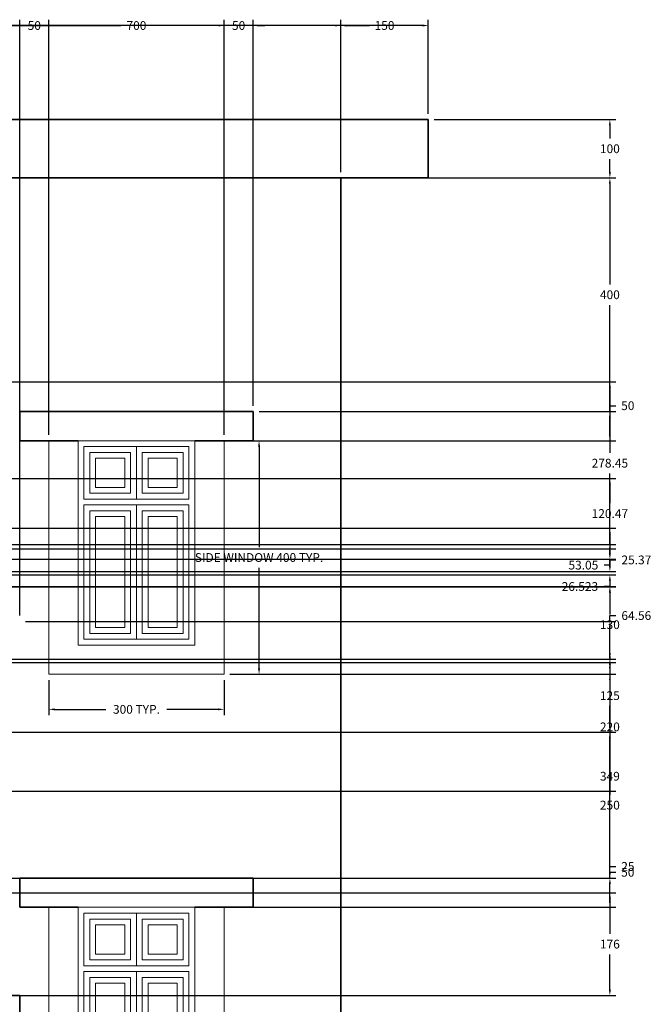
# Model space of a CAD drawing. Units: millimetres. Extents: x 937 to 4561, y 2711 to 5748.
# Tile 8 of 8: x 3479 to 4561, y 4062 to 5748. Entities that reach past the tile are written whole.
import ezdxf

# ---------------------------------------------------------------- set-up
doc = ezdxf.new("R2010")
doc.units = ezdxf.units.MM
doc.header["$MEASUREMENT"] = 0
for name, color, linetype, lineweight in [('A-ANNO-DIMS', 2, 'Continuous', 18), ('A-ELEV', 7, 'Continuous', 35), ('A-GLAZ', 4, 'Continuous', 18)]:
    doc.layers.add(name, color=color, linetype=linetype, lineweight=lineweight)
doc.styles.get("Standard").update_dxf_attribs({"font": 'arial.ttf'})
doc.dimstyles.get("Standard").update_dxf_attribs({"dimtxt": 15, "dimasz": 10, "dimexe": 10, "dimexo": 10, "dimgap": 10, "dimtad": 0, "dimtih": 1, "dimtoh": 1, "dimdec": 0, "dimzin": 0, "dimdsep": 46, "dimtxsty": 'Standard', "dimcen": 5, "dimadec": 0, "dimazin": 0, "dimtfac": 1, "dimtdec": 0, "dimtofl": 0, "dimtmove": 0, "dimatfit": 3, "dimfxl": 1, "dimtolj": 1, "dimtzin": 0, "dimarcsym": 0})

# ---------------------------------------------------------------- blocks, each defined once
blk = doc.blocks.new('WIN-SIDE')
for p, q in [((3529.5, 5026.9), (3529.5, 4626.9)), ((3579.5, 5026.9), (3779.5, 5026.9)), ((3579.5, 4676.9), (3579.5, 5026.9)), ((3779.5, 5026.9), (3779.5, 4676.9)), ((3829.5, 4626.9), (3829.5, 5026.9)), ((3779.5, 4676.9), (3579.5, 4676.9)), ((3529.5, 4626.9), (3829.5, 4626.9))]:
    blk.add_line(p, q)
for points in [[(3589.5, 5016.9), (3679.5, 5016.9), (3679.5, 4926.9), (3589.5, 4926.9)], [(3679.5, 5016.9), (3769.5, 5016.9), (3769.5, 4926.9), (3679.5, 4926.9)], [(3599.5, 5006.9), (3669.5, 5006.9), (3669.5, 4936.9), (3599.5, 4936.9)], [(3609.5, 4996.9), (3659.5, 4996.9), (3659.5, 4946.9), (3609.5, 4946.9)], [(3689.5, 5006.9), (3759.5, 5006.9), (3759.5, 4936.9), (3689.5, 4936.9)], [(3699.5, 4996.9), (3749.5, 4996.9), (3749.5, 4946.9), (3699.5, 4946.9)], [(3589.5, 4916.9), (3679.5, 4916.9), (3679.5, 4686.9), (3589.5, 4686.9)], [(3599.5, 4906.9), (3669.5, 4906.9), (3669.5, 4696.9), (3599.5, 4696.9)], [(3679.5, 4916.9), (3769.5, 4916.9), (3769.5, 4686.9), (3679.5, 4686.9)], [(3689.5, 4906.9), (3759.5, 4906.9), (3759.5, 4696.9), (3689.5, 4696.9)], [(3609.5, 4896.9), (3659.5, 4896.9), (3659.5, 4706.9), (3609.5, 4706.9)], [(3699.5, 4896.9), (3749.5, 4896.9), (3749.5, 4706.9), (3699.5, 4706.9)]]:
    blk.add_lwpolyline(points, close=True)
blk = doc.blocks.new('*D2')
at = {"layer": 'A-ANNO-DIMS', "color": 0, "lineweight": -2, "transparency": 16777216}
for p, q in [((3839.5, 5026.9), (3899.5, 5026.9)), ((3889.5, 5016.9), (3889.5, 4844.7)), ((3889.5, 4636.9), (3889.5, 4809.1)), ((3839.5, 4626.9), (3899.5, 4626.9))]:
    blk.add_line(p, q, dxfattribs=at)
at = {"layer": 'A-ANNO-DIMS', "color": 0, "transparency": 16777216}
for points in [[(3887.8, 5016.9), (3891.2, 5016.9), (3889.5, 5026.9)], [(3887.8, 4636.9), (3891.2, 4636.9), (3889.5, 4626.9)]]:
    blk.add_solid(points, dxfattribs=at)
at = {"layer": 'Defpoints', "color": 0, "transparency": 16777216}
for p in [(3829.5, 5026.9), (3889.5, 5026.9), (3829.5, 4626.9)]:
    blk.add_point(p, dxfattribs=at)
at = {"layer": 'A-ANNO-DIMS', "color": 0, "transparency": 16777216, "insert": (3889.5, 4826.9), "char_height": 15, "attachment_point": 5}
blk.add_mtext('\\A1;SIDE WINDOW 400 TYP.', dxfattribs=at)
blk = doc.blocks.new('*D3')
at = {"layer": 'A-ANNO-DIMS', "color": 0, "lineweight": -2, "transparency": 16777216}
for p, q in [((3529.5, 4616.9), (3529.5, 4556.9)), ((3829.5, 4616.9), (3829.5, 4556.9)), ((3539.5, 4566.9), (3627.2, 4566.9)), ((3819.5, 4566.9), (3731.8, 4566.9))]:
    blk.add_line(p, q, dxfattribs=at)
at = {"layer": 'A-ANNO-DIMS', "color": 0, "transparency": 16777216}
for points in [[(3539.5, 4568.6), (3539.5, 4565.2), (3529.5, 4566.9)], [(3819.5, 4568.6), (3819.5, 4565.2), (3829.5, 4566.9)]]:
    blk.add_solid(points, dxfattribs=at)
at = {"layer": 'Defpoints', "color": 0, "transparency": 16777216}
for p in [(3529.5, 4626.9), (3829.5, 4626.9), (3829.5, 4566.9)]:
    blk.add_point(p, dxfattribs=at)
at = {"layer": 'A-ANNO-DIMS', "color": 0, "transparency": 16777216, "insert": (3679.5, 4566.9), "char_height": 15, "attachment_point": 5}
blk.add_mtext('\\A1;300 TYP.', dxfattribs=at)
blk = doc.blocks.new('*D15')
at = {"layer": 'A-ANNO-DIMS', "color": 0, "lineweight": -2, "transparency": 16777216}
for p, q in [((1329.5, 4086.9), (1329.5, 5747.9)), ((1339.5, 5737.9), (2722, 5737.9)), ((4169.5, 5737.9), (2787, 5737.9)), ((4179.5, 5586.9), (4179.5, 5747.9))]:
    blk.add_line(p, q, dxfattribs=at)
at = {"layer": 'A-ANNO-DIMS', "color": 0, "transparency": 16777216}
for points in [[(1339.5, 5739.6), (1339.5, 5736.2), (1329.5, 5737.9)], [(4169.5, 5739.6), (4169.5, 5736.2), (4179.5, 5737.9)]]:
    blk.add_solid(points, dxfattribs=at)
at = {"layer": 'Defpoints', "color": 0, "transparency": 16777216}
for p in [(4179.5, 5737.9), (4179.5, 5576.9), (1329.5, 4076.9)]:
    blk.add_point(p, dxfattribs=at)
at = {"layer": 'A-ANNO-DIMS', "color": 0, "transparency": 16777216, "insert": (2754.5, 5737.9), "char_height": 15, "attachment_point": 5}
blk.add_mtext('\\A1;2850', dxfattribs=at)
blk = doc.blocks.new('*D18')
at = {"layer": 'A-ANNO-DIMS', "color": 0, "lineweight": -2, "transparency": 16777216}
for p, q in [((3329.5, 5486.9), (3329.5, 5747.9)), ((3339.5, 5737.9), (3653, 5737.9)), ((4019.5, 5737.9), (3706, 5737.9)), ((4029.5, 5486.9), (4029.5, 5747.9))]:
    blk.add_line(p, q, dxfattribs=at)
at = {"layer": 'A-ANNO-DIMS', "color": 0, "transparency": 16777216}
for points in [[(3339.5, 5739.6), (3339.5, 5736.2), (3329.5, 5737.9)], [(4019.5, 5739.6), (4019.5, 5736.2), (4029.5, 5737.9)]]:
    blk.add_solid(points, dxfattribs=at)
at = {"layer": 'Defpoints', "color": 0, "transparency": 16777216}
for p in [(4029.5, 5737.9), (3329.5, 5476.9), (4029.5, 5476.9)]:
    blk.add_point(p, dxfattribs=at)
at = {"layer": 'A-ANNO-DIMS', "color": 0, "transparency": 16777216, "insert": (3679.5, 5737.9), "char_height": 15, "attachment_point": 5}
blk.add_mtext('\\A1;700', dxfattribs=at)
blk = doc.blocks.new('*D19')
at = {"layer": 'A-ANNO-DIMS', "color": 0, "lineweight": -2, "transparency": 16777216}
for p, q in [((4029.5, 5486.9), (4029.5, 5747.9)), ((4039.5, 5737.9), (4078.6, 5737.9)), ((4169.5, 5737.9), (4130.3, 5737.9)), ((4179.5, 5586.9), (4179.5, 5747.9))]:
    blk.add_line(p, q, dxfattribs=at)
at = {"layer": 'A-ANNO-DIMS', "color": 0, "transparency": 16777216}
for points in [[(4039.5, 5739.6), (4039.5, 5736.2), (4029.5, 5737.9)], [(4169.5, 5739.6), (4169.5, 5736.2), (4179.5, 5737.9)]]:
    blk.add_solid(points, dxfattribs=at)
at = {"layer": 'Defpoints', "color": 0, "transparency": 16777216}
for p in [(4179.5, 5737.9), (4179.5, 5576.9), (4029.5, 5476.9)]:
    blk.add_point(p, dxfattribs=at)
at = {"layer": 'A-ANNO-DIMS', "color": 0, "transparency": 16777216, "insert": (4104.5, 5737.9), "char_height": 15, "attachment_point": 5}
blk.add_mtext('\\A1;150', dxfattribs=at)
blk = doc.blocks.new('*D23')
at = {"layer": 'A-ANNO-DIMS', "color": 0, "lineweight": -2, "transparency": 16777216}
for p, q in [((3029.5, 4886.9), (3029.5, 5747.9)), ((3039.5, 5737.9), (3227.6, 5737.9)), ((3469.5, 5737.9), (3281.3, 5737.9)), ((3479.5, 4727.5), (3479.5, 5747.9))]:
    blk.add_line(p, q, dxfattribs=at)
at = {"layer": 'A-ANNO-DIMS', "color": 0, "transparency": 16777216}
for points in [[(3039.5, 5739.6), (3039.5, 5736.2), (3029.5, 5737.9)], [(3469.5, 5739.6), (3469.5, 5736.2), (3479.5, 5737.9)]]:
    blk.add_solid(points, dxfattribs=at)
at = {"layer": 'Defpoints', "color": 0, "transparency": 16777216}
for p in [(3479.5, 5737.9), (3029.5, 4876.9), (3479.5, 4717.5)]:
    blk.add_point(p, dxfattribs=at)
at = {"layer": 'A-ANNO-DIMS', "color": 0, "transparency": 16777216, "insert": (3254.5, 5737.9), "char_height": 15, "attachment_point": 5}
blk.add_mtext('\\A1;450', dxfattribs=at)
blk = doc.blocks.new('*D25')
at = {"layer": 'A-ANNO-DIMS', "color": 0, "lineweight": -2, "transparency": 16777216}
for p, q in [((3469.5, 5737.9), (3459.5, 5737.9)), ((3479.5, 5086.9), (3479.5, 5747.9)), ((3529.5, 5036.9), (3529.5, 5747.9)), ((3539.5, 5737.9), (3549.5, 5737.9))]:
    blk.add_line(p, q, dxfattribs=at)
at = {"layer": 'A-ANNO-DIMS', "color": 0, "transparency": 16777216}
for points in [[(3469.5, 5739.6), (3469.5, 5736.2), (3479.5, 5737.9)], [(3539.5, 5739.6), (3539.5, 5736.2), (3529.5, 5737.9)]]:
    blk.add_solid(points, dxfattribs=at)
at = {"layer": 'Defpoints', "color": 0, "transparency": 16777216}
for p in [(3529.5, 5737.9), (3479.5, 5076.9), (3529.5, 5026.9)]:
    blk.add_point(p, dxfattribs=at)
at = {"layer": 'A-ANNO-DIMS', "color": 0, "transparency": 16777216, "insert": (3504.5, 5737.9), "char_height": 15, "attachment_point": 5}
blk.add_mtext('\\A1;50', dxfattribs=at)
blk = doc.blocks.new('*D26')
at = {"layer": 'A-ANNO-DIMS', "color": 0, "lineweight": -2, "transparency": 16777216}
for p, q in [((3819.5, 5737.9), (3809.5, 5737.9)), ((3829.5, 5036.9), (3829.5, 5747.9)), ((3879.5, 5086.9), (3879.5, 5747.9)), ((3889.5, 5737.9), (3899.5, 5737.9))]:
    blk.add_line(p, q, dxfattribs=at)
at = {"layer": 'A-ANNO-DIMS', "color": 0, "transparency": 16777216}
for points in [[(3819.5, 5739.6), (3819.5, 5736.2), (3829.5, 5737.9)], [(3889.5, 5739.6), (3889.5, 5736.2), (3879.5, 5737.9)]]:
    blk.add_solid(points, dxfattribs=at)
at = {"layer": 'Defpoints', "color": 0, "transparency": 16777216}
for p in [(3879.5, 5737.9), (3879.5, 5076.9), (3829.5, 5026.9)]:
    blk.add_point(p, dxfattribs=at)
at = {"layer": 'A-ANNO-DIMS', "color": 0, "transparency": 16777216, "insert": (3854.5, 5737.9), "char_height": 15, "attachment_point": 5}
blk.add_mtext('\\A1;50', dxfattribs=at)
blk = doc.blocks.new('*D68')
at = {"layer": 'A-ANNO-DIMS', "color": 0, "lineweight": -2, "transparency": 16777216}
for p, q in [((4490.5, 4812.8), (4490.5, 4822.8)), ((4490.5, 4822.8), (4500.5, 4822.8)), ((1364.5, 4802.8), (4500.5, 4802.8)), ((1364.5, 4777.4), (4500.5, 4777.4)), ((4490.5, 4767.4), (4490.5, 4757.4))]:
    blk.add_line(p, q, dxfattribs=at)
at = {"layer": 'A-ANNO-DIMS', "color": 0, "transparency": 16777216}
for points in [[(4488.8, 4812.8), (4492.2, 4812.8), (4490.5, 4802.8)], [(4488.8, 4767.4), (4492.2, 4767.4), (4490.5, 4777.4)]]:
    blk.add_solid(points, dxfattribs=at)
at = {"layer": 'Defpoints', "color": 0, "transparency": 16777216}
for p in [(1354.5, 4802.8), (4490.5, 4802.8), (1354.5, 4777.4)]:
    blk.add_point(p, dxfattribs=at)
at = {"layer": 'A-ANNO-DIMS', "color": 0, "transparency": 16777216, "insert": (4535.9, 4822.8), "char_height": 15, "attachment_point": 5}
blk.add_mtext('\\A1;25.37', dxfattribs=at)
blk = doc.blocks.new('*D69')
at = {"layer": 'A-ANNO-DIMS', "color": 0, "lineweight": -2, "transparency": 16777216}
for p, q in [((2957.4, 5127.7), (4500.5, 5127.7)), ((4490.5, 5117.7), (4490.5, 5006.1)), ((4490.5, 4859.2), (4490.5, 4970.8)), ((1339.5, 4849.2), (4500.5, 4849.2))]:
    blk.add_line(p, q, dxfattribs=at)
at = {"layer": 'A-ANNO-DIMS', "color": 0, "transparency": 16777216}
for points in [[(4488.8, 5117.7), (4492.2, 5117.7), (4490.5, 5127.7)], [(4488.8, 4859.2), (4492.2, 4859.2), (4490.5, 4849.2)]]:
    blk.add_solid(points, dxfattribs=at)
at = {"layer": 'Defpoints', "color": 0, "transparency": 16777216}
for p in [(2947.4, 5127.7), (4490.5, 5127.7), (1329.5, 4849.2)]:
    blk.add_point(p, dxfattribs=at)
at = {"layer": 'A-ANNO-DIMS', "color": 0, "transparency": 16777216, "insert": (4490.5, 4988.5), "char_height": 15, "attachment_point": 5}
blk.add_mtext('\\A1;278.45', dxfattribs=at)
blk = doc.blocks.new('*D75')
at = {"layer": 'A-ANNO-DIMS', "color": 0, "lineweight": -2, "transparency": 16777216}
for p, q in [((1829.5, 4646.9), (4500.5, 4646.9)), ((4490.5, 4636.9), (4490.5, 4554.6)), ((4490.5, 4436.9), (4490.5, 4519.2)), ((1829.5, 4426.9), (4500.5, 4426.9))]:
    blk.add_line(p, q, dxfattribs=at)
at = {"layer": 'A-ANNO-DIMS', "color": 0, "transparency": 16777216}
for points in [[(4488.8, 4636.9), (4492.2, 4636.9), (4490.5, 4646.9)], [(4488.8, 4436.9), (4492.2, 4436.9), (4490.5, 4426.9)]]:
    blk.add_solid(points, dxfattribs=at)
at = {"layer": 'Defpoints', "color": 0, "transparency": 16777216}
for p in [(1819.5, 4646.9), (4490.5, 4646.9), (1819.5, 4426.9)]:
    blk.add_point(p, dxfattribs=at)
at = {"layer": 'A-ANNO-DIMS', "color": 0, "transparency": 16777216, "insert": (4490.5, 4536.9), "char_height": 15, "attachment_point": 5}
blk.add_mtext('\\A1;220', dxfattribs=at)
blk = doc.blocks.new('*D76')
at = {"layer": 'A-ANNO-DIMS', "color": 0, "lineweight": -2, "transparency": 16777216}
for p, q in [((1829.5, 4776.9), (4500.5, 4776.9)), ((4490.5, 4766.9), (4490.5, 4729.6)), ((4490.5, 4656.9), (4490.5, 4694.2)), ((1829.5, 4646.9), (4500.5, 4646.9))]:
    blk.add_line(p, q, dxfattribs=at)
at = {"layer": 'A-ANNO-DIMS', "color": 0, "transparency": 16777216}
for points in [[(4488.8, 4766.9), (4492.2, 4766.9), (4490.5, 4776.9)], [(4488.8, 4656.9), (4492.2, 4656.9), (4490.5, 4646.9)]]:
    blk.add_solid(points, dxfattribs=at)
at = {"layer": 'Defpoints', "color": 0, "transparency": 16777216}
for p in [(1819.5, 4776.9), (4490.5, 4776.9), (1819.5, 4646.9)]:
    blk.add_point(p, dxfattribs=at)
at = {"layer": 'A-ANNO-DIMS', "color": 0, "transparency": 16777216, "insert": (4490.5, 4711.9), "char_height": 15, "attachment_point": 5}
blk.add_mtext('\\A1;130', dxfattribs=at)
blk = doc.blocks.new('*D78')
at = {"layer": 'A-ANNO-DIMS', "color": 0, "lineweight": -2, "transparency": 16777216}
for p, q in [((2439.5, 4962.4), (4500.5, 4962.4)), ((4490.5, 4952.4), (4490.5, 4919.9)), ((4490.5, 4852), (4490.5, 4884.5)), ((1739.5, 4842), (4500.5, 4842))]:
    blk.add_line(p, q, dxfattribs=at)
at = {"layer": 'A-ANNO-DIMS', "color": 0, "transparency": 16777216}
for points in [[(4488.8, 4952.4), (4492.2, 4952.4), (4490.5, 4962.4)], [(4488.8, 4852), (4492.2, 4852), (4490.5, 4842)]]:
    blk.add_solid(points, dxfattribs=at)
at = {"layer": 'Defpoints', "color": 0, "transparency": 16777216}
for p in [(2429.5, 4962.4), (4490.5, 4962.4), (1729.5, 4842)]:
    blk.add_point(p, dxfattribs=at)
at = {"layer": 'A-ANNO-DIMS', "color": 0, "transparency": 16777216, "insert": (4490.5, 4902.2), "char_height": 15, "attachment_point": 5}
blk.add_mtext('\\A1;120.47', dxfattribs=at)
blk = doc.blocks.new('*D80')
at = {"layer": 'A-ANNO-DIMS', "color": 0, "lineweight": -2, "transparency": 16777216}
for p, q in [((3039.5, 4876.9), (4500.5, 4876.9)), ((4490.5, 4866.9), (4490.5, 4833.9)), ((3039.5, 4823.9), (4500.5, 4823.9)), ((4490.5, 4823.9), (4490.5, 4813.9)), ((4490.5, 4813.9), (4480.5, 4813.9))]:
    blk.add_line(p, q, dxfattribs=at)
at = {"layer": 'A-ANNO-DIMS', "color": 0, "transparency": 16777216}
for points in [[(4488.8, 4866.9), (4492.2, 4866.9), (4490.5, 4876.9)], [(4488.8, 4833.9), (4492.2, 4833.9), (4490.5, 4823.9)]]:
    blk.add_solid(points, dxfattribs=at)
at = {"layer": 'Defpoints', "color": 0, "transparency": 16777216}
for p in [(3029.5, 4876.9), (3029.5, 4823.9), (4490.5, 4823.9)]:
    blk.add_point(p, dxfattribs=at)
at = {"layer": 'A-ANNO-DIMS', "color": 0, "transparency": 16777216, "insert": (4445.1, 4813.9), "char_height": 15, "attachment_point": 5}
blk.add_mtext('\\A1;53.05', dxfattribs=at)
blk = doc.blocks.new('*D81')
at = {"layer": 'A-ANNO-DIMS', "color": 0, "lineweight": -2, "transparency": 16777216}
for p, q in [((4490.5, 4833.9), (4490.5, 4843.9)), ((3039.5, 4823.9), (4500.5, 4823.9)), ((3039.5, 4797.3), (4500.5, 4797.3)), ((4490.5, 4777.3), (4480.5, 4777.3)), ((4490.5, 4787.3), (4490.5, 4777.3))]:
    blk.add_line(p, q, dxfattribs=at)
at = {"layer": 'A-ANNO-DIMS', "color": 0, "transparency": 16777216}
for points in [[(4488.8, 4833.9), (4492.2, 4833.9), (4490.5, 4823.9)], [(4488.8, 4787.3), (4492.2, 4787.3), (4490.5, 4797.3)]]:
    blk.add_solid(points, dxfattribs=at)
at = {"layer": 'Defpoints', "color": 0, "transparency": 16777216}
for p in [(3029.5, 4823.9), (3029.5, 4797.3), (4490.5, 4797.3)]:
    blk.add_point(p, dxfattribs=at)
at = {"layer": 'A-ANNO-DIMS', "color": 0, "transparency": 16777216, "insert": (4439.2, 4777.3), "char_height": 15, "attachment_point": 5}
blk.add_mtext('\\A1;26.523', dxfattribs=at)
blk = doc.blocks.new('*D88')
at = {"layer": 'A-ANNO-DIMS', "color": 0, "lineweight": -2, "transparency": 16777216}
for p, q in [((3339.5, 4252.9), (4500.5, 4252.9)), ((4490.5, 4242.9), (4490.5, 4182.6)), ((4490.5, 4086.9), (4490.5, 4147.2)), ((3339.5, 4076.9), (4500.5, 4076.9))]:
    blk.add_line(p, q, dxfattribs=at)
at = {"layer": 'A-ANNO-DIMS', "color": 0, "transparency": 16777216}
for points in [[(4488.8, 4242.9), (4492.2, 4242.9), (4490.5, 4252.9)], [(4488.8, 4086.9), (4492.2, 4086.9), (4490.5, 4076.9)]]:
    blk.add_solid(points, dxfattribs=at)
at = {"layer": 'Defpoints', "color": 0, "transparency": 16777216}
for p in [(3329.5, 4252.9), (4490.5, 4252.9), (3329.5, 4076.9)]:
    blk.add_point(p, dxfattribs=at)
at = {"layer": 'A-ANNO-DIMS', "color": 0, "transparency": 16777216, "insert": (4490.5, 4164.9), "char_height": 15, "attachment_point": 5}
blk.add_mtext('\\A1;176', dxfattribs=at)
blk = doc.blocks.new('*D89')
at = {"layer": 'A-ANNO-DIMS', "color": 0, "lineweight": -2, "transparency": 16777216}
for p, q in [((4490.5, 4287.9), (4490.5, 4297.9)), ((4490.5, 4297.9), (4500.5, 4297.9)), ((3339.5, 4277.9), (4500.5, 4277.9)), ((3339.5, 4252.9), (4500.5, 4252.9)), ((4490.5, 4242.9), (4490.5, 4232.9))]:
    blk.add_line(p, q, dxfattribs=at)
at = {"layer": 'A-ANNO-DIMS', "color": 0, "transparency": 16777216}
for points in [[(4488.8, 4287.9), (4492.2, 4287.9), (4490.5, 4277.9)], [(4488.8, 4242.9), (4492.2, 4242.9), (4490.5, 4252.9)]]:
    blk.add_solid(points, dxfattribs=at)
at = {"layer": 'Defpoints', "color": 0, "transparency": 16777216}
for p in [(3329.5, 4277.9), (4490.5, 4277.9), (3329.5, 4252.9)]:
    blk.add_point(p, dxfattribs=at)
at = {"layer": 'A-ANNO-DIMS', "color": 0, "transparency": 16777216, "insert": (4521.4, 4297.9), "char_height": 15, "attachment_point": 5}
blk.add_mtext('\\A1;25', dxfattribs=at)
blk = doc.blocks.new('*D90')
at = {"layer": 'A-ANNO-DIMS', "color": 0, "lineweight": -2, "transparency": 16777216}
for p, q in [((3339.5, 4527.9), (4500.5, 4527.9)), ((4490.5, 4517.9), (4490.5, 4420.6)), ((4490.5, 4287.9), (4490.5, 4385.2)), ((3339.5, 4277.9), (4500.5, 4277.9))]:
    blk.add_line(p, q, dxfattribs=at)
at = {"layer": 'A-ANNO-DIMS', "color": 0, "transparency": 16777216}
for points in [[(4488.8, 4517.9), (4492.2, 4517.9), (4490.5, 4527.9)], [(4488.8, 4287.9), (4492.2, 4287.9), (4490.5, 4277.9)]]:
    blk.add_solid(points, dxfattribs=at)
at = {"layer": 'Defpoints', "color": 0, "transparency": 16777216}
for p in [(3329.5, 4527.9), (4490.5, 4527.9), (3329.5, 4277.9)]:
    blk.add_point(p, dxfattribs=at)
at = {"layer": 'A-ANNO-DIMS', "color": 0, "transparency": 16777216, "insert": (4490.5, 4402.9), "char_height": 15, "attachment_point": 5}
blk.add_mtext('\\A1;250', dxfattribs=at)
blk = doc.blocks.new('*D91')
at = {"layer": 'A-ANNO-DIMS', "color": 0, "lineweight": -2, "transparency": 16777216}
for p, q in [((3376.9, 4652.9), (4500.5, 4652.9)), ((4490.5, 4642.9), (4490.5, 4608.1)), ((4490.5, 4537.9), (4490.5, 4572.7)), ((3339.5, 4527.9), (4500.5, 4527.9))]:
    blk.add_line(p, q, dxfattribs=at)
at = {"layer": 'A-ANNO-DIMS', "color": 0, "transparency": 16777216}
for points in [[(4488.8, 4642.9), (4492.2, 4642.9), (4490.5, 4652.9)], [(4488.8, 4537.9), (4492.2, 4537.9), (4490.5, 4527.9)]]:
    blk.add_solid(points, dxfattribs=at)
at = {"layer": 'Defpoints', "color": 0, "transparency": 16777216}
for p in [(3366.9, 4652.9), (4490.5, 4652.9), (3329.5, 4527.9)]:
    blk.add_point(p, dxfattribs=at)
at = {"layer": 'A-ANNO-DIMS', "color": 0, "transparency": 16777216, "insert": (4490.5, 4590.4), "char_height": 15, "attachment_point": 5}
blk.add_mtext('\\A1;125', dxfattribs=at)
blk = doc.blocks.new('*D92')
at = {"layer": 'A-ANNO-DIMS', "color": 0, "lineweight": -2, "transparency": 16777216}
for p, q in [((4490.5, 4717.5), (4490.5, 4727.5)), ((4490.5, 4727.5), (4500.5, 4727.5)), ((3489.5, 4717.5), (4500.5, 4717.5)), ((4490.5, 4662.9), (4490.5, 4707.5)), ((3376.9, 4652.9), (4500.5, 4652.9))]:
    blk.add_line(p, q, dxfattribs=at)
at = {"layer": 'A-ANNO-DIMS', "color": 0, "transparency": 16777216}
for points in [[(4488.8, 4707.5), (4492.2, 4707.5), (4490.5, 4717.5)], [(4488.8, 4662.9), (4492.2, 4662.9), (4490.5, 4652.9)]]:
    blk.add_solid(points, dxfattribs=at)
at = {"layer": 'Defpoints', "color": 0, "transparency": 16777216}
for p in [(3479.5, 4717.5), (4490.5, 4717.5), (3366.9, 4652.9)]:
    blk.add_point(p, dxfattribs=at)
at = {"layer": 'A-ANNO-DIMS', "color": 0, "transparency": 16777216, "insert": (4535.8, 4727.5), "char_height": 15, "attachment_point": 5}
blk.add_mtext('\\A1;64.56', dxfattribs=at)
blk = doc.blocks.new('*D103')
at = {"layer": 'A-ANNO-DIMS', "color": 0, "lineweight": -2, "transparency": 16777216}
for p, q in [((4490.5, 4277.9), (4490.5, 4287.9)), ((4490.5, 4287.9), (4500.5, 4287.9)), ((3889.5, 4277.9), (4500.5, 4277.9)), ((4490.5, 4237.9), (4490.5, 4267.9)), ((3839.5, 4227.9), (4500.5, 4227.9))]:
    blk.add_line(p, q, dxfattribs=at)
at = {"layer": 'A-ANNO-DIMS', "color": 0, "transparency": 16777216}
for points in [[(4488.8, 4267.9), (4492.2, 4267.9), (4490.5, 4277.9)], [(4488.8, 4237.9), (4492.2, 4237.9), (4490.5, 4227.9)]]:
    blk.add_solid(points, dxfattribs=at)
at = {"layer": 'Defpoints', "color": 0, "transparency": 16777216}
for p in [(3879.5, 4277.9), (4490.5, 4277.9), (3829.5, 4227.9)]:
    blk.add_point(p, dxfattribs=at)
at = {"layer": 'A-ANNO-DIMS', "color": 0, "transparency": 16777216, "insert": (4521.2, 4287.9), "char_height": 15, "attachment_point": 5}
blk.add_mtext('\\A1;50', dxfattribs=at)
blk = doc.blocks.new('*D104')
at = {"layer": 'A-ANNO-DIMS', "color": 0, "lineweight": -2, "transparency": 16777216}
for p, q in [((3839.5, 4626.9), (4500.5, 4626.9)), ((4490.5, 4616.9), (4490.5, 4470.1)), ((4490.5, 4287.9), (4490.5, 4434.7)), ((3889.5, 4277.9), (4500.5, 4277.9))]:
    blk.add_line(p, q, dxfattribs=at)
at = {"layer": 'A-ANNO-DIMS', "color": 0, "transparency": 16777216}
for points in [[(4488.8, 4616.9), (4492.2, 4616.9), (4490.5, 4626.9)], [(4488.8, 4287.9), (4492.2, 4287.9), (4490.5, 4277.9)]]:
    blk.add_solid(points, dxfattribs=at)
at = {"layer": 'Defpoints', "color": 0, "transparency": 16777216}
for p in [(3829.5, 4626.9), (4490.5, 4626.9), (3879.5, 4277.9)]:
    blk.add_point(p, dxfattribs=at)
at = {"layer": 'A-ANNO-DIMS', "color": 0, "transparency": 16777216, "insert": (4490.5, 4452.4), "char_height": 15, "attachment_point": 5}
blk.add_mtext('\\A1;349', dxfattribs=at)
blk = doc.blocks.new('*D105')
at = {"layer": 'A-ANNO-DIMS', "color": 0, "lineweight": -2, "transparency": 16777216}
for p, q in [((3889.5, 5076.9), (4500.5, 5076.9)), ((4490.5, 5076.9), (4490.5, 5086.9)), ((4490.5, 5086.9), (4500.5, 5086.9)), ((4490.5, 5036.9), (4490.5, 5066.9)), ((3839.5, 5026.9), (4500.5, 5026.9))]:
    blk.add_line(p, q, dxfattribs=at)
at = {"layer": 'A-ANNO-DIMS', "color": 0, "transparency": 16777216}
for points in [[(4488.8, 5066.9), (4492.2, 5066.9), (4490.5, 5076.9)], [(4488.8, 5036.9), (4492.2, 5036.9), (4490.5, 5026.9)]]:
    blk.add_solid(points, dxfattribs=at)
at = {"layer": 'Defpoints', "color": 0, "transparency": 16777216}
for p in [(3879.5, 5076.9), (4490.5, 5076.9), (3829.5, 5026.9)]:
    blk.add_point(p, dxfattribs=at)
at = {"layer": 'A-ANNO-DIMS', "color": 0, "transparency": 16777216, "insert": (4521.2, 5086.9), "char_height": 15, "attachment_point": 5}
blk.add_mtext('\\A1;50', dxfattribs=at)
blk = doc.blocks.new('*D106')
at = {"layer": 'A-ANNO-DIMS', "color": 0, "lineweight": -2, "transparency": 16777216}
for p, q in [((4039.5, 5476.9), (4500.5, 5476.9)), ((4490.5, 5466.9), (4490.5, 5294.6)), ((4490.5, 5086.9), (4490.5, 5259.2)), ((3889.5, 5076.9), (4500.5, 5076.9))]:
    blk.add_line(p, q, dxfattribs=at)
at = {"layer": 'A-ANNO-DIMS', "color": 0, "transparency": 16777216}
for points in [[(4488.8, 5466.9), (4492.2, 5466.9), (4490.5, 5476.9)], [(4488.8, 5086.9), (4492.2, 5086.9), (4490.5, 5076.9)]]:
    blk.add_solid(points, dxfattribs=at)
at = {"layer": 'Defpoints', "color": 0, "transparency": 16777216}
for p in [(4029.5, 5476.9), (4490.5, 5476.9), (3879.5, 5076.9)]:
    blk.add_point(p, dxfattribs=at)
at = {"layer": 'A-ANNO-DIMS', "color": 0, "transparency": 16777216, "insert": (4490.5, 5276.9), "char_height": 15, "attachment_point": 5}
blk.add_mtext('\\A1;400', dxfattribs=at)
blk = doc.blocks.new('*D107')
at = {"layer": 'A-ANNO-DIMS', "color": 0, "lineweight": -2, "transparency": 16777216}
for p, q in [((4189.5, 5576.9), (4500.5, 5576.9)), ((4490.5, 5566.9), (4490.5, 5544.6)), ((4490.5, 5486.9), (4490.5, 5509.2)), ((4039.5, 5476.9), (4500.5, 5476.9))]:
    blk.add_line(p, q, dxfattribs=at)
at = {"layer": 'A-ANNO-DIMS', "color": 0, "transparency": 16777216}
for points in [[(4488.8, 5566.9), (4492.2, 5566.9), (4490.5, 5576.9)], [(4488.8, 5486.9), (4492.2, 5486.9), (4490.5, 5476.9)]]:
    blk.add_solid(points, dxfattribs=at)
at = {"layer": 'Defpoints', "color": 0, "transparency": 16777216}
for p in [(4179.5, 5576.9), (4490.5, 5576.9), (4029.5, 5476.9)]:
    blk.add_point(p, dxfattribs=at)
at = {"layer": 'A-ANNO-DIMS', "color": 0, "transparency": 16777216, "insert": (4490.5, 5526.9), "char_height": 15, "attachment_point": 5}
blk.add_mtext('\\A1;100', dxfattribs=at)

msp = doc.modelspace()

# ---------------------------------------------------------------- linework, layer by layer
at = {"layer": 'A-ELEV'}
for p, q in [((3929.4852, 5576.9013), (3179.4852, 5576.9013)), ((4179.4852, 5576.9013), (3929.4852, 5576.9013)), ((4179.4852, 5476.9013), (4179.4852, 5576.9013)), ((3179.4852, 5476.9013), (4179.4852, 5476.9013)), ((4029.4852, 3076.9013), (4029.4852, 5476.9013)), ((3479.4852, 5026.9013), (3479.4852, 5076.9013)), ((3479.4852, 5076.9013), (3879.4852, 5076.9013)), ((3879.4852, 5076.9013), (3879.4852, 5026.9013)), ((3579.4852, 5026.9013), (3479.4852, 5026.9013)), ((3879.4852, 5026.9013), (3779.4852, 5026.9013)), ((3479.4852, 4227.9001), (3479.4852, 4277.9001)), ((3479.4852, 4277.9001), (3879.4852, 4277.9001)), ((3879.4852, 4277.9001), (3879.4852, 4227.9001)), ((3579.4852, 4227.9001), (3479.4852, 4227.9001)), ((3879.4852, 4227.9001), (3779.4852, 4227.9001)), ((1429.4852, 4076.9013), (3479.4852, 4076.9013)), ((3329.4852, 4076.9013), (3479.4852, 4076.9013)), ((3479.4852, 4076.9013), (3479.4852, 3976.9013))]:
    msp.add_line(p, q, dxfattribs=at)

# ---------------------------------------------------------------- block references
at = {"layer": 'A-GLAZ'}
for p in [(0, 0), (0, -799.0013)]:
    msp.add_blockref('WIN-SIDE', p, dxfattribs=at)

# ---------------------------------------------------------------- dimensions: what is measured, and where the dimension line sits
at = {"layer": 'A-ANNO-DIMS'}
for base, p1, p2, picture, middle in [((4179.4852, 5737.9013), (1329.4852, 4076.9013), (4179.4852, 5576.9013), '*D15', (2754.4852, 5737.9013)), ((3479.4852, 5737.9013), (3029.4852, 4876.9013), (3479.4852, 4717.4604), '*D23', (3254.4852, 5737.9013)), ((4029.4852, 5737.9013), (3329.4852, 5476.9013), (4029.4852, 5476.9013), '*D18', (3679.4852, 5737.9013)), ((3529.4852, 5737.9013), (3479.4852, 5076.9013), (3529.4852, 5026.9013), '*D25', (3504.4852, 5737.9013)), ((3879.4852, 5737.9013), (3829.4852, 5026.9013), (3879.4852, 5076.9013), '*D26', (3854.4852, 5737.9013)), ((4179.4852, 5737.9013), (4029.4852, 5476.9013), (4179.4852, 5576.9013), '*D19', (4104.4852, 5737.9013))]:
    dim = msp.add_linear_dim(base=base, p1=p1, p2=p2, dimstyle='Standard', override={"dimdec": 0, "dimlfac": 1, "dimrnd": 0, "dimzin": 0, "dimdsep": 46, "dimlunit": 2}, dxfattribs=at)
    dim.commit()
    dim.dimension.update_dxf_attribs({"geometry": picture, "text_midpoint": middle})
for base, p1, p2, override, picture, middle in [((4490.4852, 5576.9013), (4029.4852, 5476.9013), (4179.4852, 5576.9013), {"dimdec": 0, "dimlfac": 1, "dimrnd": 0, "dimzin": 0, "dimdsep": 46, "dimlunit": 2}, '*D107', (4490.4852, 5526.9013)), ((4490.4852, 5476.9013), (3879.4852, 5076.9013), (4029.4852, 5476.9013), {"dimdec": 0, "dimlfac": 1, "dimrnd": 0, "dimzin": 0, "dimdsep": 46, "dimlunit": 2}, '*D106', (4490.4852, 5276.9013)), ((4490.4852, 5127.6834), (1329.4852, 4849.2371), (2947.4456, 5127.6834), {"dimdec": 2, "dimlfac": 1, "dimrnd": 0, "dimzin": 0, "dimdsep": 46, "dimlunit": 2}, '*D69', (4490.4852, 4988.4602)), ((4490.4852, 5076.9013), (3829.4852, 5026.9013), (3879.4852, 5076.9013), {"dimdec": 0, "dimlfac": 1, "dimrnd": 0, "dimzin": 0, "dimdsep": 46, "dimlunit": 2}, '*D105', (4521.2031, 5086.9013)), ((4490.4852, 4962.4414), (1729.4852, 4841.9734), (2429.4852, 4962.4414), {"dimdec": 2, "dimlfac": 1, "dimrnd": 0, "dimzin": 0, "dimdsep": 46, "dimlunit": 2}, '*D78', (4490.4852, 4902.2074)), ((4490.4852, 4823.8556), (3029.4852, 4876.9013), (3029.4852, 4823.8556), {"dimdec": 2, "dimlfac": 1, "dimrnd": 0, "dimzin": 0, "dimdsep": 46, "dimlunit": 2}, '*D80', (4445.1203, 4813.8556)), ((4490.4852, 4797.3328), (3029.4852, 4823.8556), (3029.4852, 4797.3328), {"dimdec": 3, "dimlfac": 1, "dimrnd": 0, "dimzin": 0, "dimdsep": 46, "dimlunit": 2}, '*D81', (4439.2216, 4777.3328)), ((4490.4852, 4802.8045), (1354.4852, 4777.437), (1354.4852, 4802.8045), {"dimdec": 2, "dimlfac": 1, "dimrnd": 0, "dimzin": 0, "dimdsep": 46, "dimlunit": 2}, '*D68', (4535.9218, 4822.8045)), ((4490.4852, 4776.9013), (1819.4852, 4646.9013), (1819.4852, 4776.9013), {"dimdec": 0, "dimlfac": 1, "dimrnd": 0, "dimzin": 0, "dimdsep": 46, "dimlunit": 2}, '*D76', (4490.4852, 4711.9013)), ((4490.4852, 4717.4604), (3366.9387, 4652.9001), (3479.4852, 4717.4604), {"dimdec": 2, "dimlfac": 1, "dimrnd": 0, "dimzin": 0, "dimdsep": 46, "dimlunit": 2}, '*D92', (4535.8297, 4727.4604)), ((4490.4852, 4646.9013), (1819.4852, 4426.9013), (1819.4852, 4646.9013), {"dimdec": 0, "dimlfac": 1, "dimrnd": 0, "dimzin": 0, "dimdsep": 46, "dimlunit": 2}, '*D75', (4490.4852, 4536.9013)), ((4490.4852, 4652.9001), (3329.4852, 4527.9001), (3366.9387, 4652.9001), {"dimdec": 0, "dimlfac": 1, "dimrnd": 0, "dimzin": 0, "dimdsep": 46, "dimlunit": 2}, '*D91', (4490.4852, 4590.4001)), ((4490.4852, 4626.9013), (3879.4852, 4277.9001), (3829.4852, 4626.9013), {"dimdec": 0, "dimlfac": 1, "dimrnd": 0, "dimzin": 0, "dimdsep": 46, "dimlunit": 2}, '*D104', (4490.4852, 4452.4007)), ((4490.4852, 4527.9001), (3329.4852, 4277.9001), (3329.4852, 4527.9001), {"dimdec": 0, "dimlfac": 1, "dimrnd": 0, "dimzin": 0, "dimdsep": 46, "dimlunit": 2}, '*D90', (4490.4852, 4402.9001)), ((4490.4852, 4277.9001), (3329.4852, 4252.9001), (3329.4852, 4277.9001), {"dimdec": 0, "dimlfac": 1, "dimrnd": 0, "dimzin": 0, "dimdsep": 46, "dimlunit": 2}, '*D89', (4521.4129, 4297.9001)), ((4490.4852, 4277.9001), (3829.4852, 4227.9001), (3879.4852, 4277.9001), {"dimdec": 0, "dimlfac": 1, "dimrnd": 0, "dimzin": 0, "dimdsep": 46, "dimlunit": 2}, '*D103', (4521.2031, 4287.9001)), ((4490.4852, 4252.9001), (3329.4852, 4076.9013), (3329.4852, 4252.9001), {"dimdec": 0, "dimlfac": 1, "dimrnd": 0, "dimzin": 0, "dimdsep": 46, "dimlunit": 2}, '*D88', (4490.4852, 4164.9007))]:
    dim = msp.add_linear_dim(base=base, p1=p1, p2=p2, angle=90, dimstyle='Standard', override=override, dxfattribs=at)
    dim.commit()
    dim.dimension.update_dxf_attribs({"geometry": picture, "text_midpoint": middle})
dim = msp.add_linear_dim(base=(3889.4852, 5026.9013), p1=(3829.4852, 4626.9013), p2=(3829.4852, 5026.9013), angle=90, text='SIDE WINDOW <> TYP.', dimstyle='Standard', override={"dimdec": 0, "dimlfac": 1, "dimrnd": 0, "dimzin": 0, "dimdsep": 46, "dimlunit": 2}, dxfattribs=at)
dim.commit()
dim.dimension.update_dxf_attribs({"geometry": '*D2', "text_midpoint": (3889.4852, 4826.9013)})
dim = msp.add_linear_dim(base=(3829.4852, 4566.9013), p1=(3529.4852, 4626.9013), p2=(3829.4852, 4626.9013), text='<> TYP.', dimstyle='Standard', override={"dimdec": 0, "dimlfac": 1, "dimrnd": 0, "dimzin": 0, "dimdsep": 46, "dimlunit": 2}, dxfattribs=at)
dim.commit()
dim.dimension.update_dxf_attribs({"geometry": '*D3', "text_midpoint": (3679.4852, 4566.9013)})

doc.saveas('drawing.dxf')
